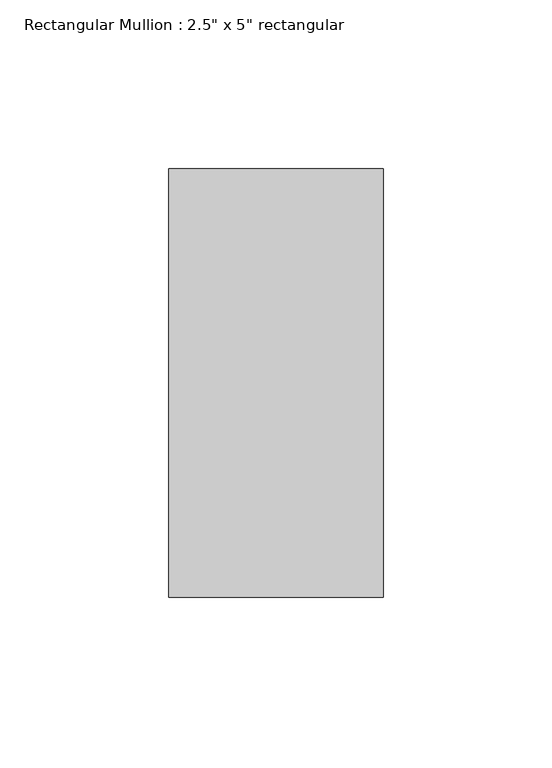
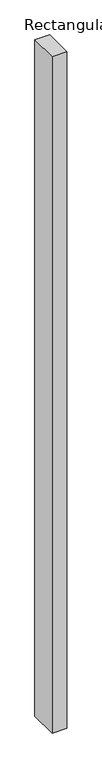
"""IFC4 building model written with IfcOpenShell, lengths in millimetres: member geometry."""

from ifc_helpers import new_model, si_unit, frame, origin, place, context, project, spatial, polyline, outline, extrude, source, transform, mapped, element, save


def member_3f395ae9(model_context):
    return source(origin(), model_context, "Body", "SweptSolid", [
        extrude(outline(polyline([(0.0, 63.5), (0.0, -63.5), (-63.5, -63.5), (-63.5, 63.5), (0.0, 63.5)])), frame((0.0, 0.0, -3048.0), z_axis=(0.0, 0.0, 1.0), x_axis=(1.0, 0.0, 0.0)), (0.0, 0.0, 1.0), 3048.0),
    ])


if __name__ == "__main__":
    model = new_model("IFC4")
    model_context = context("Model", 3, world=origin())
    ifc_project = project(units=[si_unit("LENGTHUNIT", "METRE", prefix="MILLI")], contexts=[model_context])
    site = spatial("IfcSite", under=ifc_project)
    building = spatial("IfcBuilding", under=site)
    placement = place(None, origin())
    member_shape = member_3f395ae9(model_context)
    element("IfcMember", 1, ObjectType="Rectangular Mullion : 2.5\" x 5\" rectangular", at=placement, inside=building, context=model_context, shape_type="MappedRepresentation", body=[
        mapped(member_shape, transform((0.0, 0.0, 0.0), x_axis=(1.0, 0.0, 0.0), y_axis=(0.0, 1.0, 0.0), z_axis=(0.0, 0.0, 1.0))),
    ])
    save(model, "model.ifc")

# Revit data of these elements
# Type "Rectangular Mullion : 2.5\" x 5\" rectangular"
#   built-in parameter 1007304 = 0.416667 (stored number, unit not read)
#   built-in parameter 1007301 = 0.104167 (stored number, unit not read)
#   built-in parameter 1007300 = 0.104167 (stored number, unit not read)
# Element 1 (IfcMember, "Rectangular Mullion : 2.5\" x 5\" rectangular")
#   Materials on its faces: "Aluminum"
# Materials
#   "Aluminum": class "Metal", colour RGB 247 247 247, transparency 0, Description = "Aluminum 6061", Cost = 0
